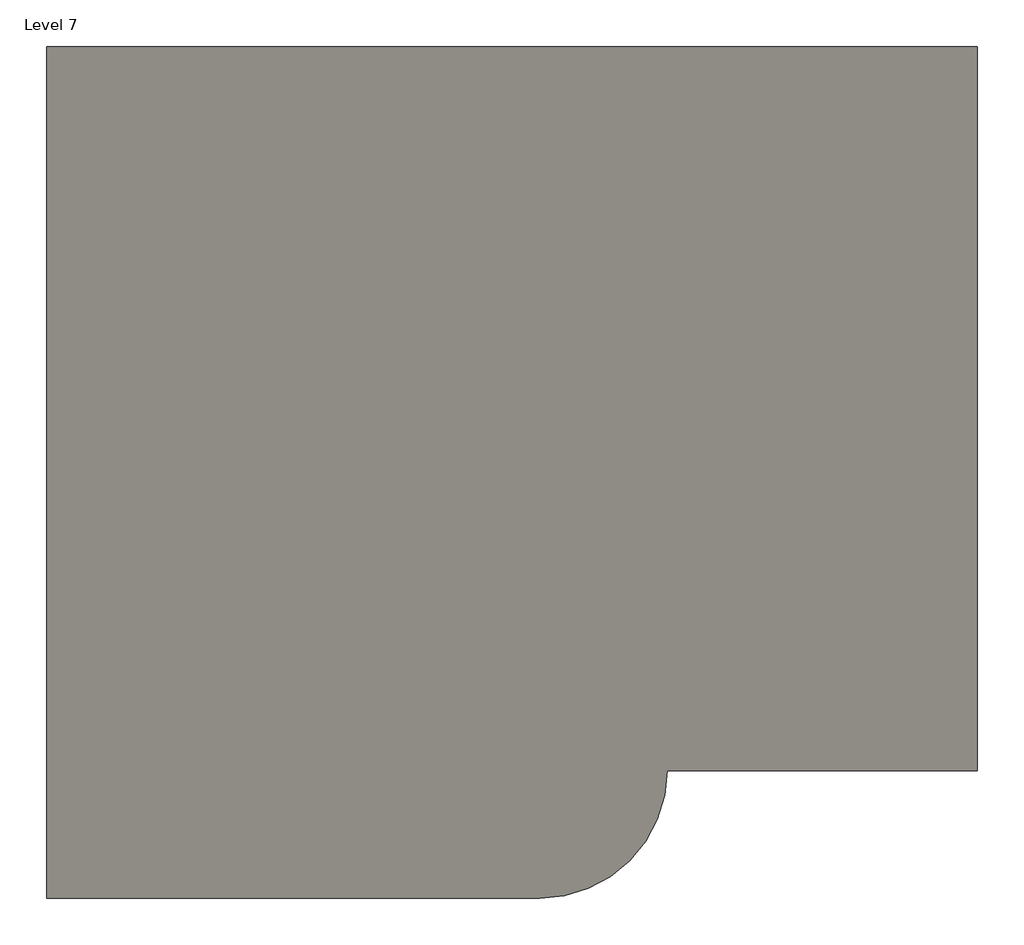
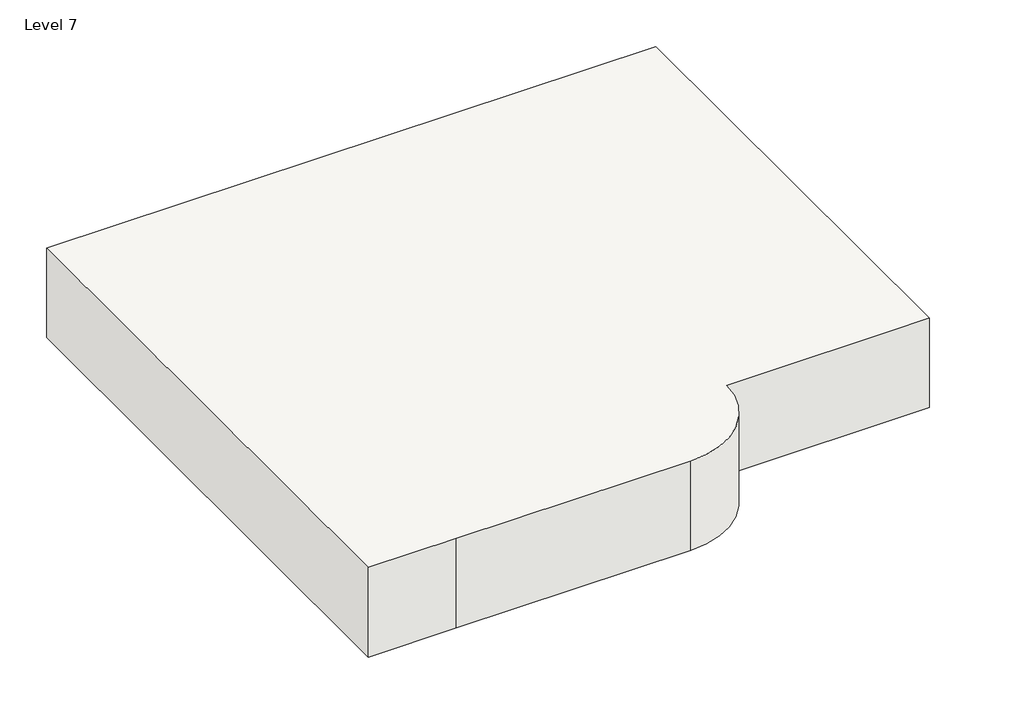
# One storey: 1 slab.
"""IFC4 building model written with IfcOpenShell, lengths in millimetres."""

from ifc_helpers import new_model, si_unit, point, frame, frame_2d, origin, place, context, project, spatial, polyline, circle_curve, trimmed, segment, composite_curve, outline, extrude, element, save

model = new_model("IFC4")

# Units and contexts
model_context = context("Model", 3, world=origin())
ifc_project = project(units=[si_unit("LENGTHUNIT", "METRE", prefix="MILLI")], contexts=[model_context])

# Site, building, storey
site = spatial("IfcSite", under=ifc_project)
building = spatial("IfcBuilding", under=site)
storey = spatial("IfcBuildingStorey", under=building, Name="Level 7", Elevation=18288.0)

# Slab
placement = place(None, origin())
element("IfcSlab", 1, ObjectType="wall design 4", at=placement, inside=storey, context=model_context, shape_type="SweptSolid", body=[
    extrude(outline(composite_curve([segment(polyline([(-5468.2104559, 11493.328737), (-5468.2104559, 825.328737), (-10040.2104559, 825.328737)]), True, "CONTINUOUS"), segment(trimmed(circle_curve(frame_2d((-11919.8104559, 825.328737)), 1879.6), [point((-10040.2104559, 825.328737))], [point((-11919.8104559, -1054.271263))], False, "CARTESIAN"), True, "CONTINUOUS"), segment(polyline([(-11919.8104559, -1054.271263), (-17203.0104559, -1054.271263), (-19184.2104559, -1054.271263), (-19184.2104559, 11493.328737), (-5468.2104559, 11493.328737)]), True, "CONTINUOUS")], self_intersect=False)), frame((0.0, 0.0, 17907.0), z_axis=(0.0, 0.0, 1.0), x_axis=(1.0, 0.0, 0.0)), (0.0, 0.0, 1.0), 2133.6),
])

save(model, "model.ifc")

# Revit data of these elements
# Type "wall design 4"
#   Assembly Code = "B1010"
#   Function = 0
#   Layers, outside or top first: 7' - 0" "Damp-proofing" (function 1)
# Element 1 (IfcSlab, "wall design 4")
#   Height Offset From Level = 5' - 9"
#   Phase Created = New Construction
#   Materials on its faces: "Damp-proofing"
# Materials
#   "Damp-proofing": class "Generic", colour RGB 127 127 127, transparency 0, Description = "Damp-proofing", Cost = 0
